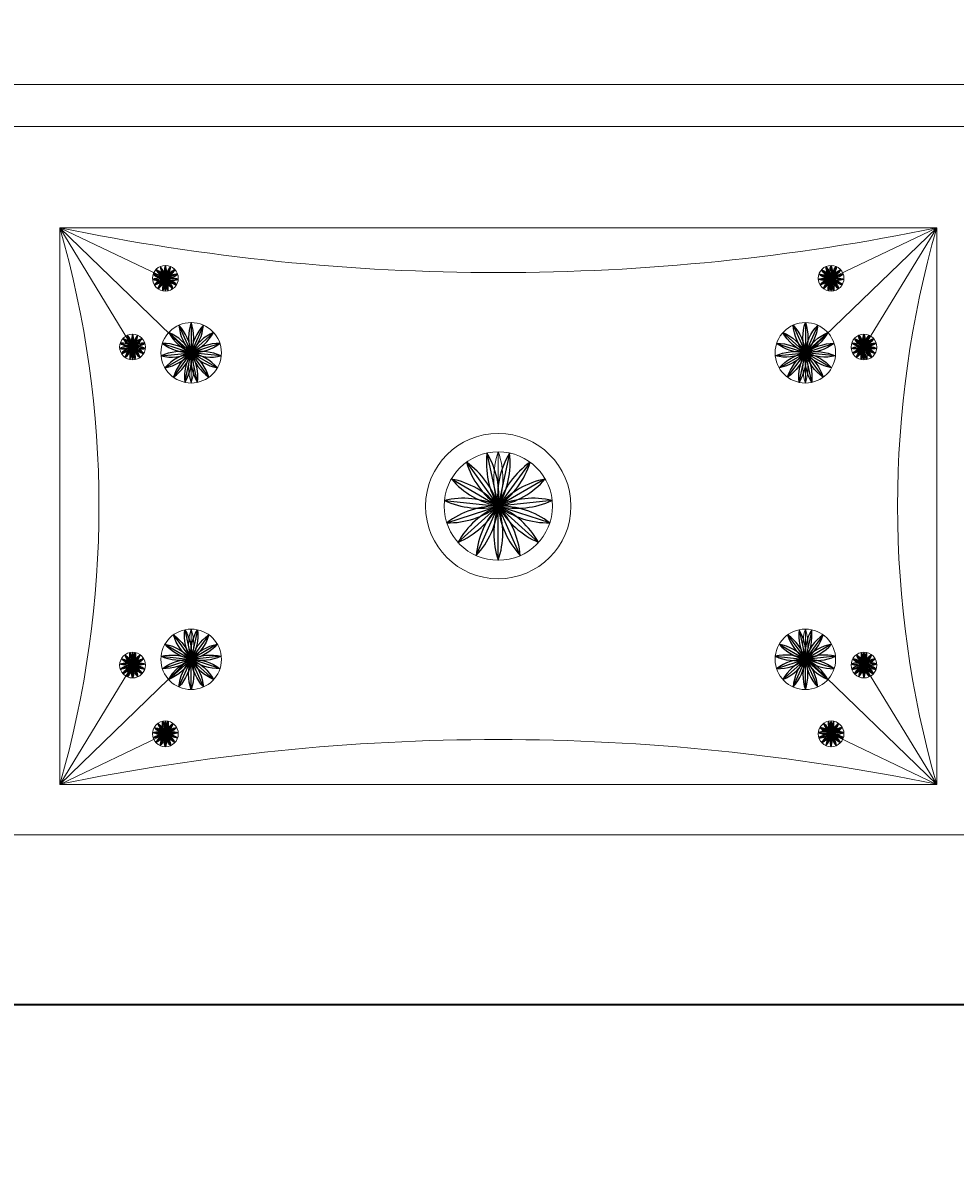
# Model space of a CAD drawing. Units: inches. Extents: x -61 to 1599, y -1316 to 257.
# Tile 7 of 204: x 149 to 175, y -1211 to -1180. Entities that reach past the tile are written whole.
import ezdxf

# ---------------------------------------------------------------- set-up
doc = ezdxf.new("R2010")
doc.units = ezdxf.units.IN
doc.header["$MEASUREMENT"] = 0
for name, color, linetype, lineweight in [('A-ANNO-DIMS', 2, 'Continuous', 18), ('FURNITURE', 83, 'Continuous', 18), ('WALLS', 4, 'Continuous', 35)]:
    doc.layers.add(name, color=color, linetype=linetype, lineweight=lineweight)
doc.layers.add('LT', color=8, linetype='Continuous')
doc.styles.get("Standard").update_dxf_attribs({"font": 'arial.ttf'})
doc.dimstyles.get("Standard").update_dxf_attribs({"dimtxt": 0.18, "dimasz": 0.18, "dimexe": 0.18, "dimexo": 0.0625, "dimgap": 0.09, "dimtad": 0, "dimtih": 1, "dimtoh": 1, "dimdec": 0, "dimzin": 0, "dimdsep": 46, "dimlunit": 3, "dimtxsty": 'Standard', "dimcen": 0.09, "dimadec": 0, "dimazin": 0, "dimtfac": 1, "dimtdec": 0, "dimtofl": 0, "dimtmove": 0, "dimatfit": 3, "dimfxl": 1, "dimtolj": 1, "dimtzin": 0, "dimarcsym": 0})

# ---------------------------------------------------------------- blocks, each defined once
blk = doc.blocks.new('*U3')
at = {"layer": 'LT'}
blk.add_line((0, 0.175), (0, -0.175), dxfattribs=at)
for centre, start, end in [((0.509, 0), 160.9983, 199.0017), ((-0.509, 0), 340.9983, 19.0017)]:
    blk.add_arc(centre, 0.539, start, end, dxfattribs=at)
blk = doc.blocks.new('*U4')
at = {"layer": 'LT', "transparency": 16777216}
for p, rotation in [((-66.605, -18.692), 48.00000000000001), ((-66.546, -18.649), 24), ((-66.404, -18.649), 336.0000000000001), ((-66.345, -18.692), 312), ((-66.649, -18.828), 96), ((-66.642, -18.755), 72), ((-66.627, -18.897), 120), ((-66.578, -18.951), 144), ((-66.512, -18.981), 168.0000000000001), ((-66.439, -18.981), 192), ((-66.372, -18.951), 216), ((-66.323, -18.897), 240), ((-66.308, -18.755), 288.0000000000001), ((-66.301, -18.828), 264)]:
    blk.add_blockref('*U3', p, dxfattribs=dict(at, rotation=rotation))
blk.add_blockref('*U3', (-66.475, -18.634), dxfattribs=at)
blk = doc.blocks.new('*U20')
at = {"layer": 'LT'}
blk.add_line((0, 0.175), (0, -0.175), dxfattribs=at)
for centre, start, end in [((0.509, 0), 160.9983, 199.0017), ((-0.509, 0), 340.9983, 19.0017)]:
    blk.add_arc(centre, 0.539, start, end, dxfattribs=at)
blk = doc.blocks.new('*U21')
at = {"layer": 'LT', "transparency": 16777216}
for p, rotation in [((-66.605, -18.692), 48.00000000000001), ((-66.546, -18.649), 24), ((-66.404, -18.649), 336.0000000000001), ((-66.345, -18.692), 312), ((-66.649, -18.828), 96), ((-66.642, -18.755), 72), ((-66.627, -18.897), 120), ((-66.578, -18.951), 144), ((-66.512, -18.981), 168.0000000000001), ((-66.439, -18.981), 192), ((-66.372, -18.951), 216), ((-66.323, -18.897), 240), ((-66.308, -18.755), 288.0000000000001), ((-66.301, -18.828), 264)]:
    blk.add_blockref('*U20', p, dxfattribs=dict(at, rotation=rotation))
blk.add_blockref('*U20', (-66.475, -18.634), dxfattribs=at)
blk = doc.blocks.new('*U52')
at = {"layer": 'LT'}
blk.add_line((0, 0.175), (0, -0.175), dxfattribs=at)
for centre, start, end in [((0.509, 0), 160.9983, 199.0017), ((-0.509, 0), 340.9983, 19.0017)]:
    blk.add_arc(centre, 0.539, start, end, dxfattribs=at)
blk = doc.blocks.new('*U53')
at = {"layer": 'LT', "transparency": 16777216}
for p, rotation in [((-66.605, -18.692), 48.00000000000001), ((-66.546, -18.649), 24), ((-66.404, -18.649), 336.0000000000001), ((-66.345, -18.692), 312), ((-66.649, -18.828), 96), ((-66.642, -18.755), 72), ((-66.627, -18.897), 120), ((-66.578, -18.951), 144), ((-66.512, -18.981), 168.0000000000001), ((-66.439, -18.981), 192), ((-66.372, -18.951), 216), ((-66.323, -18.897), 240), ((-66.308, -18.755), 288.0000000000001), ((-66.301, -18.828), 264)]:
    blk.add_blockref('*U52', p, dxfattribs=dict(at, rotation=rotation))
blk.add_blockref('*U52', (-66.475, -18.634), dxfattribs=at)
blk = doc.blocks.new('*U29')
at = {"layer": 'LT'}
blk.add_line((0, 0.175), (0, -0.175), dxfattribs=at)
for centre, start, end in [((0.509, 0), 160.9983, 199.0017), ((-0.509, 0), 340.9983, 19.0017)]:
    blk.add_arc(centre, 0.539, start, end, dxfattribs=at)
blk = doc.blocks.new('*U30')
at = {"layer": 'LT', "transparency": 16777216}
for p, rotation in [((-66.605, -18.692), 48.00000000000001), ((-66.546, -18.649), 24), ((-66.404, -18.649), 336.0000000000001), ((-66.345, -18.692), 312), ((-66.649, -18.828), 96), ((-66.642, -18.755), 72), ((-66.627, -18.897), 120), ((-66.578, -18.951), 144), ((-66.512, -18.981), 168.0000000000001), ((-66.439, -18.981), 192), ((-66.372, -18.951), 216), ((-66.323, -18.897), 240), ((-66.308, -18.755), 288.0000000000001), ((-66.301, -18.828), 264)]:
    blk.add_blockref('*U29', p, dxfattribs=dict(at, rotation=rotation))
blk.add_blockref('*U29', (-66.475, -18.634), dxfattribs=at)
blk = doc.blocks.new('*U5')
at = {"layer": 'LT'}
blk.add_line((0, 0.412), (0, -0.412), dxfattribs=at)
for centre, start, end in [((1.198, 0), 160.9983, 199.0017), ((-1.198, 0), 340.9983, 19.0017)]:
    blk.add_arc(centre, 1.267, start, end, dxfattribs=at)
blk = doc.blocks.new('*U47')
at = {"layer": 'LT', "transparency": 16777216}
for p, rotation in [((-156.501, -43.858), 24), ((-156.165, -43.858), 336.0000000000001), ((-156.725, -44.108), 72), ((-156.639, -43.959), 48.00000000000001), ((-156.027, -43.959), 312), ((-155.941, -44.108), 288.0000000000001), ((-156.743, -44.278), 96), ((-156.69, -44.441), 120), ((-156.575, -44.569), 144), ((-156.419, -44.639), 168), ((-156.247, -44.639), 192), ((-156.091, -44.569), 216), ((-155.976, -44.441), 240), ((-155.923, -44.278), 264)]:
    blk.add_blockref('*U5', p, dxfattribs=dict(at, rotation=rotation))
blk.add_blockref('*U5', (-156.333, -43.823), dxfattribs=at)
blk = doc.blocks.new('*U22')
at = {"layer": 'LT'}
blk.add_line((0, 0.412), (0, -0.412), dxfattribs=at)
for centre, start, end in [((1.198, 0), 160.9983, 199.0017), ((-1.198, 0), 340.9983, 19.0017)]:
    blk.add_arc(centre, 1.267, start, end, dxfattribs=at)
blk = doc.blocks.new('*U23')
at = {"layer": 'LT', "transparency": 16777216}
for p, rotation in [((-156.501, -43.858), 24), ((-156.165, -43.858), 336.0000000000001), ((-156.725, -44.108), 72), ((-156.639, -43.959), 48.00000000000001), ((-156.027, -43.959), 312), ((-155.941, -44.108), 288.0000000000001), ((-156.743, -44.278), 96), ((-156.69, -44.441), 120), ((-156.575, -44.569), 144), ((-156.419, -44.639), 168), ((-156.247, -44.639), 192), ((-156.091, -44.569), 216), ((-155.976, -44.441), 240), ((-155.923, -44.278), 264)]:
    blk.add_blockref('*U22', p, dxfattribs=dict(at, rotation=rotation))
blk.add_blockref('*U22', (-156.333, -43.823), dxfattribs=at)
blk = doc.blocks.new('*U54')
at = {"layer": 'LT'}
blk.add_line((0, 0.739), (0, -0.739), dxfattribs=at)
for centre, start, end in [((2.147, 0), 160.9983, 199.0017), ((-2.147, 0), 340.9983, 19.0017)]:
    blk.add_arc(centre, 2.27, start, end, dxfattribs=at)
blk = doc.blocks.new('*U41')
at = {"layer": 'LT', "transparency": 16777216}
for p, rotation in [((-280.542, -78.621), 23.99999999999999), ((-279.941, -78.621), 336.0000000000001), ((-280.791, -78.801), 48.00000000000001), ((-279.692, -78.801), 312), ((-280.945, -79.067), 72), ((-279.539, -79.067), 288.0000000000001), ((-280.977, -79.373), 96), ((-280.882, -79.665), 120), ((-279.602, -79.665), 240), ((-279.507, -79.373), 264), ((-280.676, -79.894), 144), ((-280.395, -80.019), 168), ((-280.088, -80.019), 191.9999999999999), ((-279.807, -79.894), 216)]:
    blk.add_blockref('*U54', p, dxfattribs=dict(at, rotation=rotation))
blk.add_blockref('*U54', (-280.242, -78.557), dxfattribs=at)
blk = doc.blocks.new('*U42')
at = {"layer": 'LT'}
blk.add_line((0, 0.412), (0, -0.412), dxfattribs=at)
for centre, start, end in [((1.198, 0), 160.9983, 199.0017), ((-1.198, 0), 340.9983, 19.0017)]:
    blk.add_arc(centre, 1.267, start, end, dxfattribs=at)
blk = doc.blocks.new('*U43')
at = {"layer": 'LT', "transparency": 16777216}
for p, rotation in [((-156.501, -43.858), 24), ((-156.165, -43.858), 336.0000000000001), ((-156.725, -44.108), 72), ((-156.639, -43.959), 48.00000000000001), ((-156.027, -43.959), 312), ((-155.941, -44.108), 288.0000000000001), ((-156.743, -44.278), 96), ((-156.69, -44.441), 120), ((-156.575, -44.569), 144), ((-156.419, -44.639), 168), ((-156.247, -44.639), 192), ((-156.091, -44.569), 216), ((-155.976, -44.441), 240), ((-155.923, -44.278), 264)]:
    blk.add_blockref('*U42', p, dxfattribs=dict(at, rotation=rotation))
blk.add_blockref('*U42', (-156.333, -43.823), dxfattribs=at)
blk = doc.blocks.new('*U31')
at = {"layer": 'LT'}
blk.add_line((0, 0.412), (0, -0.412), dxfattribs=at)
for centre, start, end in [((1.198, 0), 160.9983, 199.0017), ((-1.198, 0), 340.9983, 19.0017)]:
    blk.add_arc(centre, 1.267, start, end, dxfattribs=at)
blk = doc.blocks.new('*U32')
at = {"layer": 'LT', "transparency": 16777216}
for p, rotation in [((-156.501, -43.858), 24), ((-156.165, -43.858), 336.0000000000001), ((-156.725, -44.108), 72), ((-156.639, -43.959), 48.00000000000001), ((-156.027, -43.959), 312), ((-155.941, -44.108), 288.0000000000001), ((-156.743, -44.278), 96), ((-156.69, -44.441), 120), ((-156.575, -44.569), 144), ((-156.419, -44.639), 168), ((-156.247, -44.639), 192), ((-156.091, -44.569), 216), ((-155.976, -44.441), 240), ((-155.923, -44.278), 264)]:
    blk.add_blockref('*U31', p, dxfattribs=dict(at, rotation=rotation))
blk.add_blockref('*U31', (-156.333, -43.823), dxfattribs=at)
blk = doc.blocks.new('*U48')
at = {"layer": 'LT'}
blk.add_line((0, 0.175), (0, -0.175), dxfattribs=at)
for centre, start, end in [((0.509, 0), 160.9983, 199.0017), ((-0.509, 0), 340.9983, 19.0017)]:
    blk.add_arc(centre, 0.539, start, end, dxfattribs=at)
blk = doc.blocks.new('*U49')
at = {"layer": 'LT', "transparency": 16777216}
for p, rotation in [((-66.605, -18.692), 48.00000000000001), ((-66.546, -18.649), 24), ((-66.404, -18.649), 336.0000000000001), ((-66.345, -18.692), 312), ((-66.649, -18.828), 96), ((-66.642, -18.755), 72), ((-66.627, -18.897), 120), ((-66.578, -18.951), 144), ((-66.512, -18.981), 168.0000000000001), ((-66.439, -18.981), 192), ((-66.372, -18.951), 216), ((-66.323, -18.897), 240), ((-66.308, -18.755), 288.0000000000001), ((-66.301, -18.828), 264)]:
    blk.add_blockref('*U48', p, dxfattribs=dict(at, rotation=rotation))
blk.add_blockref('*U48', (-66.475, -18.634), dxfattribs=at)
blk = doc.blocks.new('*U24')
at = {"layer": 'LT'}
blk.add_line((0, 0.175), (0, -0.175), dxfattribs=at)
for centre, start, end in [((0.509, 0), 160.9983, 199.0017), ((-0.509, 0), 340.9983, 19.0017)]:
    blk.add_arc(centre, 0.539, start, end, dxfattribs=at)
blk = doc.blocks.new('*U25')
at = {"layer": 'LT', "transparency": 16777216}
for p, rotation in [((-66.605, -18.692), 48.00000000000001), ((-66.546, -18.649), 24), ((-66.404, -18.649), 336.0000000000001), ((-66.345, -18.692), 312), ((-66.649, -18.828), 96), ((-66.642, -18.755), 72), ((-66.627, -18.897), 120), ((-66.578, -18.951), 144), ((-66.512, -18.981), 168.0000000000001), ((-66.439, -18.981), 192), ((-66.372, -18.951), 216), ((-66.323, -18.897), 240), ((-66.308, -18.755), 288.0000000000001), ((-66.301, -18.828), 264)]:
    blk.add_blockref('*U24', p, dxfattribs=dict(at, rotation=rotation))
blk.add_blockref('*U24', (-66.475, -18.634), dxfattribs=at)
blk = doc.blocks.new('*U50')
at = {"layer": 'LT'}
blk.add_line((0, 0.175), (0, -0.175), dxfattribs=at)
for centre, start, end in [((0.509, 0), 160.9983, 199.0017), ((-0.509, 0), 340.9983, 19.0017)]:
    blk.add_arc(centre, 0.539, start, end, dxfattribs=at)
blk = doc.blocks.new('*U51')
at = {"layer": 'LT', "transparency": 16777216}
for p, rotation in [((-66.605, -18.692), 48.00000000000001), ((-66.546, -18.649), 24), ((-66.404, -18.649), 336.0000000000001), ((-66.345, -18.692), 312), ((-66.649, -18.828), 96), ((-66.642, -18.755), 72), ((-66.627, -18.897), 120), ((-66.578, -18.951), 144), ((-66.512, -18.981), 168.0000000000001), ((-66.439, -18.981), 192), ((-66.372, -18.951), 216), ((-66.323, -18.897), 240), ((-66.308, -18.755), 288.0000000000001), ((-66.301, -18.828), 264)]:
    blk.add_blockref('*U50', p, dxfattribs=dict(at, rotation=rotation))
blk.add_blockref('*U50', (-66.475, -18.634), dxfattribs=at)
blk = doc.blocks.new('*U26')
at = {"layer": 'LT'}
blk.add_line((0, 0.175), (0, -0.175), dxfattribs=at)
for centre, start, end in [((0.509, 0), 160.9983, 199.0017), ((-0.509, 0), 340.9983, 19.0017)]:
    blk.add_arc(centre, 0.539, start, end, dxfattribs=at)
blk = doc.blocks.new('*U27')
at = {"layer": 'LT', "transparency": 16777216}
for p, rotation in [((-66.605, -18.692), 48.00000000000001), ((-66.546, -18.649), 24), ((-66.404, -18.649), 336.0000000000001), ((-66.345, -18.692), 312), ((-66.649, -18.828), 96), ((-66.642, -18.755), 72), ((-66.627, -18.897), 120), ((-66.578, -18.951), 144), ((-66.512, -18.981), 168.0000000000001), ((-66.439, -18.981), 192), ((-66.372, -18.951), 216), ((-66.323, -18.897), 240), ((-66.308, -18.755), 288.0000000000001), ((-66.301, -18.828), 264)]:
    blk.add_blockref('*U26', p, dxfattribs=dict(at, rotation=rotation))
blk.add_blockref('*U26', (-66.475, -18.634), dxfattribs=at)
blk = doc.blocks.new('BED-DOUBLE')
for p, q in [((1.272, 20.467), (70.263, 20.467)), ((1.272, 19.317), (70.263, 19.317)), ((37.147, 1.379), (37.147, 16.557)), ((61.064, 16.557), (37.147, 16.557)), ((37.147, 16.557), (40.027, 15.18)), ((37.147, 16.557), (40.715, 13.107)), ((37.147, 16.557), (39.13, 13.305)), ((61.064, 16.557), (57.496, 13.107)), ((61.064, 16.557), (58.185, 15.18)), ((61.064, 16.557), (59.081, 13.305)), ((40.027, 15.18), (40.027, 14.829)), ((58.185, 15.18), (58.185, 14.829)), ((39.13, 13.305), (39.13, 12.955)), ((40.729, 13.149), (40.729, 12.324)), ((57.483, 13.149), (57.483, 12.324)), ((59.081, 13.305), (59.081, 12.955)), ((49.106, 8.968), (49.106, 10.447)), ((40.729, 4.788), (40.729, 5.613)), ((57.483, 4.788), (57.483, 5.613)), ((39.13, 4.631), (39.13, 4.982)), ((59.081, 4.631), (59.081, 4.982)), ((37.147, 1.379), (40.715, 4.83)), ((61.064, 1.379), (57.496, 4.83)), ((37.147, 1.379), (39.13, 4.631)), ((61.064, 1.379), (59.081, 4.631)), ((40.027, 2.756), (40.027, 3.107)), ((58.185, 2.756), (58.185, 3.107)), ((37.147, 1.379), (40.027, 2.756)), ((61.064, 1.379), (58.185, 2.756)), ((61.064, 1.379), (61.064, 1.379))]:
    blk.add_line(p, q)
for points in [[(1.272, 88.537), (1.272, 3.449, 0.414214), (4.722, 0), (66.813, 0, 0.414214), (70.263, 3.449), (70.263, 88.537, 0.414214), (66.813, 91.987), (4.722, 91.987, 0.414214)], [(40.027, 15.18, 0.167358), (40.027, 14.829, 0.167358)], [(39.13, 13.305, 0.167358), (39.13, 12.955, 0.167358)], [(40.729, 13.149, 0.167358), (40.729, 12.324, 0.167358)], [(57.483, 12.324, 0.167358), (57.483, 13.149, 0.167358)], [(59.081, 12.955, 0.167358), (59.081, 13.305, 0.167358)], [(49.106, 8.968, 0.167358), (49.106, 10.447, 0.167358)], [(40.729, 5.613, 0.167358), (40.729, 4.788, 0.167358)], [(57.483, 4.788, 0.167358), (57.483, 5.613, 0.167358)], [(39.13, 4.982, 0.167358), (39.13, 4.631, 0.167358)], [(59.081, 4.631, 0.167358), (59.081, 4.982, 0.167358)], [(40.027, 3.107, 0.167358), (40.027, 2.756, 0.167358)], [(58.185, 2.756, 0.167358), (58.185, 3.107, 0.167358)]]:
    blk.add_lwpolyline(points, format="xyb", close=True)
blk.add_lwpolyline([(61.064, 16.557), (61.064, 1.379), (37.147, 1.379)])
for centre, radius in [((40.027, 15.18), 0.351), ((58.185, 15.18), 0.351), ((40.729, 13.149), 0.825), ((57.483, 13.149), 0.825), ((39.13, 13.305), 0.351), ((59.081, 13.305), 0.351), ((49.106, 8.968), 1.982), ((49.106, 8.968), 1.478), ((40.729, 4.788), 0.825), ((57.483, 4.788), 0.825), ((39.13, 4.631), 0.351), ((59.081, 4.631), 0.351), ((40.027, 2.756), 0.351), ((58.185, 2.756), 0.351)]:
    blk.add_circle(centre, radius)
for centre, radius, start, end in [((10.674, 8.968), 27.54, 344.0046, 15.9954), ((49.106, 74.54), 59.203, 258.34678, 281.65322), ((87.538, 8.968), 27.54, 164.0046, 195.9954), ((58.694, 15.005), 0.539, 160.9983, 199.0017), ((57.675, 15.005), 0.539, 340.9983, 19.0017), ((49.106, -56.603), 59.203, 78.34678, 101.65322)]:
    blk.add_arc(centre, radius, start, end)
for name, p in [('*U30', (106.502, 33.99)), ('*U23', (197.062, 57.384)), ('*U21', (105.605, 32.115))]:
    blk.add_blockref(name, p)
at = {"extrusion": (0, 0, -1), "zscale": -1}
for name, p in [('*U25', (8.291, 33.99)), ('*U32', (98.85, 57.384)), ('*U27', (7.394, 32.115))]:
    blk.add_blockref(name, p, dxfattribs=at)
at = {"rotation": 180}
for name, p in [('*U41', (-231.136, -70.328)), ('*U43', (-98.85, -39.447)), ('*U51', (-7.394, -14.178)), ('*U49', (-8.291, -16.053))]:
    blk.add_blockref(name, p, dxfattribs=at)
at = {"extrusion": (0, 0, -1), "zscale": -1, "rotation": 180}
for name, p in [('*U47', (-197.062, -39.447)), ('*U4', (-105.605, -14.178)), ('*U53', (-106.502, -16.053))]:
    blk.add_blockref(name, p, dxfattribs=at)
blk = doc.blocks.new('*D635')
at = {"layer": 'A-ANNO-DIMS', "color": 0, "lineweight": -2, "transparency": 16777216}
for p, q in [((111.872, -1202.381), (111.872, -1216.391)), ((183.57, -1202.381), (183.57, -1216.391)), ((112.052, -1216.211), (147.193, -1216.211)), ((183.39, -1216.211), (148.248, -1216.211))]:
    blk.add_line(p, q, dxfattribs=at)
at = {"layer": 'A-ANNO-DIMS', "color": 0, "transparency": 16777216}
for points in [[(112.052, -1216.181), (112.052, -1216.241), (111.872, -1216.211)], [(183.39, -1216.181), (183.39, -1216.241), (183.57, -1216.211)]]:
    blk.add_solid(points, dxfattribs=at)
at = {"layer": 'DEFPOINTS', "color": 0, "transparency": 16777216}
for p in [(111.872, -1202.318), (183.57, -1202.318), (183.57, -1216.211)]:
    blk.add_point(p, dxfattribs=at)
at = {"layer": 'A-ANNO-DIMS', "color": 0, "transparency": 16777216, "insert": (147.721, -1216.211), "char_height": 0.18, "attachment_point": 5}
blk.add_mtext('\\A1;72 TYP.', dxfattribs=at)
blk = doc.blocks.new('*D687')
at = {"layer": 'A-ANNO-DIMS', "color": 0, "lineweight": -2, "transparency": 16777216}
for p, q in [((289.418, 181.677), (-61.077, 181.677)), ((-60.897, 181.497), (-60.897, -528.952)), ((-60.897, -1239.765), (-60.897, -529.316)), ((319.64, -1239.945), (-61.077, -1239.945))]:
    blk.add_line(p, q, dxfattribs=at)
at = {"layer": 'A-ANNO-DIMS', "color": 0, "transparency": 16777216}
for points in [[(-60.927, 181.497), (-60.867, 181.497), (-60.897, 181.677)], [(-60.927, -1239.765), (-60.867, -1239.765), (-60.897, -1239.945)]]:
    blk.add_solid(points, dxfattribs=at)
at = {"layer": 'DEFPOINTS', "color": 0, "transparency": 16777216}
for p in [(289.481, 181.677), (-60.897, -1239.945), (319.703, -1239.945)]:
    blk.add_point(p, dxfattribs=at)
at = {"layer": 'A-ANNO-DIMS', "color": 0, "transparency": 16777216, "insert": (-60.897, -529.134), "char_height": 0.18, "attachment_point": 5}
blk.add_mtext('\\A1;1421.6', dxfattribs=at)

msp = doc.modelspace()

# ---------------------------------------------------------------- linework, layer by layer
at = {"layer": 'WALLS'}
msp.add_line((14.7028, -1206.9446), (237.7028, -1206.9446), dxfattribs=at)

# ---------------------------------------------------------------- block references
at = {"layer": 'FURNITURE'}
msp.add_blockref('BED-DOUBLE', (113.2612, -1202.3177), dxfattribs=at)

# ---------------------------------------------------------------- dimensions: what is measured, and where the dimension line sits
at = {"layer": 'A-ANNO-DIMS'}
dim = msp.add_linear_dim(base=(-60.8972, -1239.9446), p1=(289.4807, 181.6771), p2=(319.7028, -1239.9446), angle=90, dimstyle='Standard', override={"dimdec": 1, "dimlfac": 1, "dimrnd": 0, "dimzin": 0, "dimdsep": 46, "dimlunit": 2}, dxfattribs=at)
dim.commit()
dim.dimension.update_dxf_attribs({"geometry": '*D687', "text_midpoint": (-60.8972, -529.1337)})
dim = msp.add_linear_dim(base=(183.5695, -1216.2111), p1=(111.8719, -1202.3182), p2=(183.5695, -1202.3182), text='<> TYP.', dimstyle='Standard', override={"dimdec": 0, "dimlfac": 1, "dimrnd": 0, "dimzin": 0, "dimdsep": 46, "dimlunit": 2}, dxfattribs=at)
dim.commit()
dim.dimension.update_dxf_attribs({"geometry": '*D635', "text_midpoint": (147.7207, -1216.2111)})

doc.saveas('drawing.dxf')
